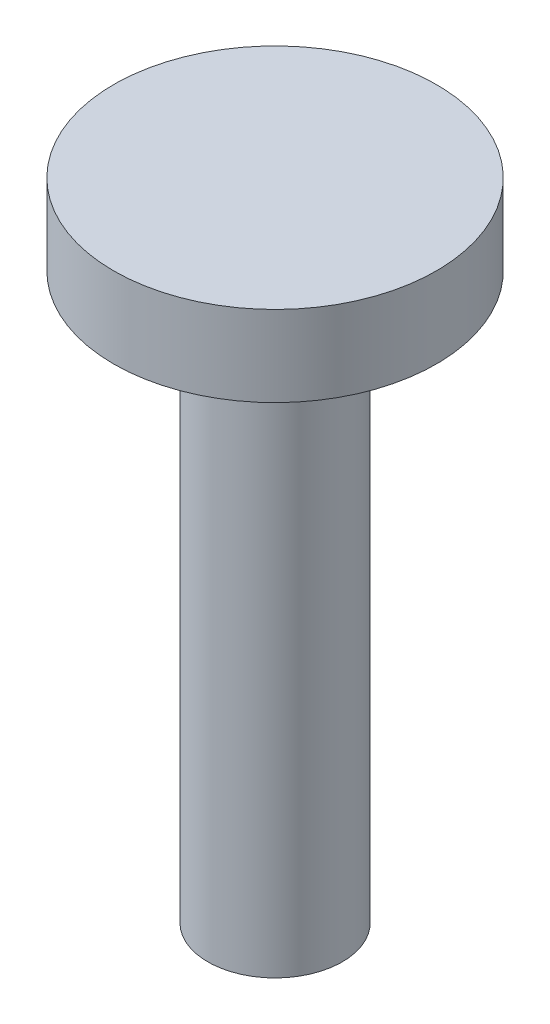
from build123d import *

# Parameters (mm, degrees)
SHANK_PROFILE_5_R = 2.5
SHANK_5X21_DEPTH  = 10.5
HEAD_PROFILE_12_R = 6
HEAD_12X3_DEPTH   = 3


with BuildPart() as part:
    # Shank Profile Ø5 → Shank Ø5x21 (new, symmetric)
    with BuildSketch(Plane(origin=(0, 0, 0), x_dir=(1, 0, 0), z_dir=(0, 1, 0))):
        with Locations(Location((0, 0, 0), (0, 0, 90))):
            Circle(SHANK_PROFILE_5_R)
    extrude(amount=SHANK_5X21_DEPTH, both=True)

    # Head Profile Ø12 → Head Ø12x3 (add)
    with BuildSketch(Plane(origin=(0, 10.5, 0), x_dir=(1, 0, 0), z_dir=(0, 1, 0))):
        with Locations(Location((0, 0, 0), (0, 0, 270))):
            Circle(HEAD_PROFILE_12_R)
    extrude(amount=HEAD_12X3_DEPTH)


solid = part.part
